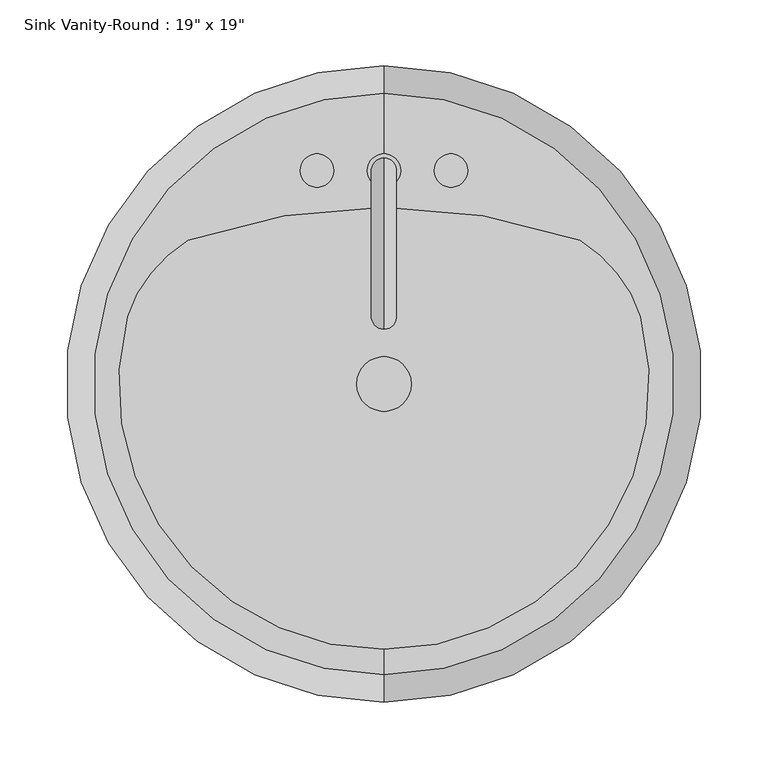
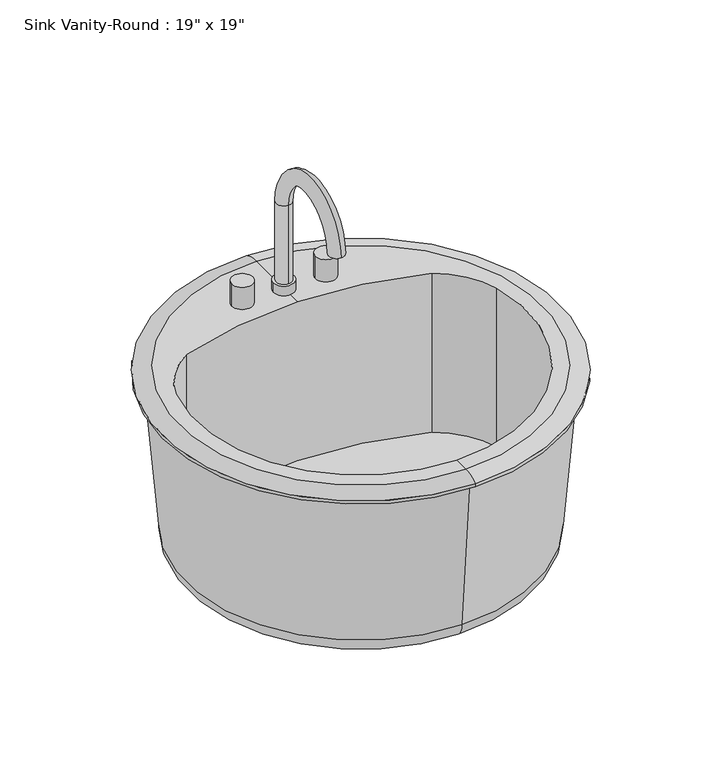
"""IFC4 building model written with IfcOpenShell, lengths in millimetres: flow terminal geometry."""

from ifc_helpers import new_model, si_unit, point, frame, frame_2d, origin, place, context, project, spatial, polyline, circle_curve, ellipse_curve, trimmed, segment, composite_curve, outline, extrude, source, transform, mapped, element, save
from ifc_brep_helpers import plane_surface, cylinder_surface, revolved_surface, advanced_brep


def flow_terminal_d49f872f(model_context):
    return source(origin(), model_context, "Body", "SolidModel", [
        advanced_brep(
        [(83.9517406, 247.0927185, 796.925), (109.3517406, 247.0927185, 796.925), (96.6517406, 237.5677185, 909.6375), (96.6517406, 256.6177185, 909.6375), (96.6517406, 256.6177185, 809.1602909), (96.6517406, 237.5677185, 809.1602909), (96.6517406, 145.7775038, 909.6375), (96.6517406, 126.7275038, 909.6375), (83.9517406, 247.0927185, 809.1602909), (109.3517406, 247.0927185, 809.1602909)],
        [
            (0, 1, circle_curve(frame((96.6517406, 247.0927185, 796.925), z_axis=(0.0, 0.0, -1.0), x_axis=(1.0, 0.0, 0.0)), 12.7)),
            (1, 0, circle_curve(frame((96.6517406, 247.0927185, 796.925), z_axis=(0.0, 0.0, -1.0), x_axis=(1.0, 0.0, 0.0)), 12.7)),
            (2, 3, circle_curve(frame((96.6517406, 247.0927185, 909.6375), z_axis=(0.0, 0.0, -1.0), x_axis=(0.0, 1.0, 0.0)), 9.525)),
            (3, 4),
            (4, 5, circle_curve(frame((96.6517406, 247.0927185, 809.1602909), z_axis=(0.0, 0.0, 1.0), x_axis=(0.0, 1.0, 0.0)), 9.525)),
            (5, 2),
            (3, 2, circle_curve(frame((96.6517406, 247.0927185, 909.6375), z_axis=(0.0, 0.0, -1.0), x_axis=(0.0, 1.0, 0.0)), 9.525)),
            (5, 4, circle_curve(frame((96.6517406, 247.0927185, 809.1602909), z_axis=(0.0, 0.0, 1.0), x_axis=(0.0, 1.0, 0.0)), 9.525)),
            (6, 7, circle_curve(frame((96.6517406, 136.2525038, 909.6375), z_axis=(0.0, 0.0, -1.0), x_axis=(0.0, -1.0, 0.0)), 9.525)),
            (7, 6, circle_curve(frame((96.6517406, 136.2525038, 909.6375), z_axis=(0.0, 0.0, -1.0), x_axis=(0.0, -1.0, 0.0)), 9.525)),
            (2, 6, circle_curve(frame((96.6517406, 191.6726112, 909.6375), z_axis=(1.0, 0.0, 0.0), x_axis=(0.0, 1.0, 0.0)), 45.8951073)),
            (7, 3, circle_curve(frame((96.6517406, 191.6726112, 909.6375), z_axis=(-1.0, 0.0, 0.0), x_axis=(0.0, 1.0, 0.0)), 64.9451073)),
            (8, 9, circle_curve(frame((96.6517406, 247.0927185, 809.1602909), z_axis=(0.0, 0.0, 1.0), x_axis=(1.0, 0.0, 0.0)), 12.7)),
            (9, 8, circle_curve(frame((96.6517406, 247.0927185, 809.1602909), z_axis=(0.0, 0.0, 1.0), x_axis=(1.0, 0.0, 0.0)), 12.7)),
            (8, 0),
            (1, 9),
        ],
        [
            plane_surface(frame((96.6517406, 237.5677185, 796.925), z_axis=(0.0, 0.0, -1.0), x_axis=(1.0, 0.0, 0.0))),
            cylinder_surface(frame((96.6517406, 247.0927185, 796.925), z_axis=(0.0, 0.0, -1.0), x_axis=(0.0, 1.0, 0.0)), 9.525),
            plane_surface(frame((96.6517406, 191.6726112, 909.6375), z_axis=(0.0, 0.0, -1.0), x_axis=(0.0, -1.0, 0.0))),
            revolved_surface(trimmed(ellipse_curve(frame((96.6517406, 247.0927185, 909.6375), z_axis=(0.0, 0.0, -1.0), x_axis=(0.0, 1.0, 0.0)), 9.525, 9.525), [point((96.6517406, 237.5677185, 909.6375))], [point((96.6517406, 256.6177185, 909.6375))], True, "CARTESIAN"), (96.6517406, 191.6726112, 909.6375), (1.0, 0.0, 0.0)),
            revolved_surface(trimmed(ellipse_curve(frame((96.6517406, 247.0927185, 909.6375), z_axis=(0.0, 0.0, -1.0), x_axis=(0.0, 1.0, 0.0)), 9.525, 9.525), [point((96.6517406, 256.6177185, 909.6375))], [point((96.6517406, 237.5677185, 909.6375))], True, "CARTESIAN"), (96.6517406, 191.6726112, 909.6375), (1.0, 0.0, 0.0)),
            plane_surface(frame((109.3517406, 247.0927185, 809.1602909), z_axis=(0.0, 0.0, 1.0), x_axis=(0.0, 1.0, 0.0))),
            cylinder_surface(frame((96.6517406, 247.0927185, 796.925), z_axis=(0.0, 0.0, 1.0), x_axis=(1.0, 0.0, 0.0)), 12.7),
        ],
        [
            (0, [[1, 2]]),
            (1, [[3, 4, 5, 6]]),
            (1, [[7, -6, 8, -4]]),
            (2, [[9, 10]]),
            (3, [[-3, 11, -10, 12]]),
            (4, [[-7, -12, -9, -11]]),
            (5, [[13, 14], [-5, -8]]),
            (6, [[-13, 15, -2, 16]]),
            (6, [[-14, -16, -1, -15]]),
        ],
    ),
        extrude(outline(composite_curve([segment(trimmed(circle_curve(frame_2d((45.8517406, 247.0927185)), 12.7), [point((33.1517406, 247.0927185))], [point((58.5517406, 247.0927185))], False, "CARTESIAN"), True, "CONTINUOUS"), segment(trimmed(circle_curve(frame_2d((45.8517406, 247.0927185)), 12.7), [point((58.5517406, 247.0927185))], [point((33.1517406, 247.0927185))], False, "CARTESIAN"), True, "CONTINUOUS")], self_intersect=False)), frame((0.0, 0.0, 796.925), z_axis=(0.0, 0.0, 1.0), x_axis=(1.0, 0.0, 0.0)), (0.0, 0.0, 1.0), 28.575),
        extrude(outline(composite_curve([segment(trimmed(circle_curve(frame_2d((147.4517406, 247.0927185)), 12.7), [point((134.7517406, 247.0927185))], [point((160.1517406, 247.0927185))], False, "CARTESIAN"), True, "CONTINUOUS"), segment(trimmed(circle_curve(frame_2d((147.4517406, 247.0927185)), 12.7), [point((160.1517406, 247.0927185))], [point((134.7517406, 247.0927185))], False, "CARTESIAN"), True, "CONTINUOUS")], self_intersect=False)), frame((0.0, 0.0, 796.925), z_axis=(0.0, 0.0, 1.0), x_axis=(1.0, 0.0, 0.0)), (0.0, 0.0, 1.0), 28.575),
        extrude(outline(composite_curve([segment(trimmed(circle_curve(frame_2d((96.6517406, 85.1677185)), 20.6375), [point((76.0142406, 85.1677185))], [point((117.2892406, 85.1677185))], False, "CARTESIAN"), True, "CONTINUOUS"), segment(trimmed(circle_curve(frame_2d((96.6517406, 85.1677185)), 20.6375), [point((117.2892406, 85.1677185))], [point((76.0142406, 85.1677185))], False, "CARTESIAN"), True, "CONTINUOUS")], self_intersect=False)), frame((0.0, 0.0, 571.5), z_axis=(0.0, 0.0, 1.0), x_axis=(1.0, 0.0, 0.0)), (0.0, 0.0, 1.0), 21.1842611),
        advanced_brep(
        [(96.6517406, -135.3870093, 796.925), (96.6517406, 305.7224463, 796.925), (96.6517406, 326.4677185, 791.36875), (96.6517406, -156.1322815, 791.36875), (96.6517406, -116.2405705, 796.925), (-98.1703414, 136.2525038, 796.925), (-52.1534933, 194.0861398, 796.925), (96.6517406, 219.2662048, 796.925), (245.4569744, 194.0861398, 796.925), (291.4738225, 136.2525038, 796.925), (96.6517406, -107.1264028, 571.5), (96.6517406, 277.4618398, 571.5), (96.6517406, 85.1677185, 571.5), (96.6517406, -127.6827361, 592.6842611), (96.6517406, 298.0181731, 592.6842611), (96.6517406, -144.2260315, 787.4), (96.6517406, 314.5614685, 787.4), (96.6517406, -156.1322815, 787.4), (96.6517406, 326.4677185, 787.4), (245.4569744, 194.0861398, 592.6842611), (-52.1534933, 194.0861398, 592.6842611), (-98.1703414, 136.2525038, 592.6842611), (291.4738225, 136.2525038, 592.6842611)],
        [
            (0, 1, circle_curve(frame((96.6517406, 85.1677185, 796.925), z_axis=(0.0, 0.0, -1.0), x_axis=(0.0, 1.0, 0.0)), 220.5547278)),
            (1, 2, circle_curve(frame((96.6517406, 309.4374616, 769.289434), z_axis=(-1.0, 0.0, 0.0), x_axis=(0.0, 1.0, 0.0)), 27.8841505)),
            (2, 3, circle_curve(frame((96.6517406, 85.1677185, 791.36875), z_axis=(0.0, 0.0, 1.0), x_axis=(0.0, 1.0, 0.0)), 241.3)),
            (3, 0, circle_curve(frame((96.6517406, -139.1020246, 769.289434), z_axis=(-1.0, 0.0, 0.0), x_axis=(0.0, -1.0, 0.0)), 27.8841505)),
            (1, 0, circle_curve(frame((96.6517406, 85.1677185, 796.925), z_axis=(0.0, 0.0, -1.0), x_axis=(0.0, 1.0, 0.0)), 220.5547278)),
            (3, 2, circle_curve(frame((96.6517406, 85.1677185, 791.36875), z_axis=(0.0, 0.0, 1.0), x_axis=(0.0, 1.0, 0.0)), 241.3)),
            (0, 4),
            (4, 5, circle_curve(frame((96.6517406, 85.1677185, 796.925), z_axis=(0.0, 0.0, -1.0), x_axis=(1.0, 0.0, 0.0)), 201.408289)),
            (5, 6, circle_curve(frame((1.3689689, 104.2755165, 796.925), z_axis=(0.0, 0.0, -1.0), x_axis=(1.0, 0.0, 0.0)), 104.5495194)),
            (6, 7, circle_curve(frame((96.6517406, -233.0168462, 796.925), z_axis=(0.0, 0.0, -1.0), x_axis=(1.0, 0.0, 0.0)), 452.283051)),
            (7, 1),
            (7, 8, circle_curve(frame((96.6517406, -233.0168462, 796.925), z_axis=(0.0, 0.0, -1.0), x_axis=(1.0, 0.0, 0.0)), 452.283051)),
            (8, 9, circle_curve(frame((191.9345122, 104.2755165, 796.925), z_axis=(0.0, 0.0, -1.0), x_axis=(1.0, 0.0, 0.0)), 104.5495194)),
            (9, 4, circle_curve(frame((96.6517406, 85.1677185, 796.925), z_axis=(0.0, 0.0, -1.0), x_axis=(1.0, 0.0, 0.0)), 201.408289)),
            (10, 11, circle_curve(frame((96.6517406, 85.1677185, 571.5), z_axis=(0.0, 0.0, -1.0), x_axis=(0.0, 1.0, 0.0)), 192.2941213)),
            (11, 12),
            (12, 10),
            (11, 10, circle_curve(frame((96.6517406, 85.1677185, 571.5), z_axis=(0.0, 0.0, -1.0), x_axis=(0.0, 1.0, 0.0)), 192.2941213)),
            (10, 13, circle_curve(frame((96.6517406, -107.1264028, 592.0656396), z_axis=(-1.0, 0.0, 0.0), x_axis=(0.0, -1.0, 0.0)), 20.5656396)),
            (13, 14, circle_curve(frame((96.6517406, 85.1677185, 592.6842611), z_axis=(0.0, 0.0, -1.0), x_axis=(0.0, 1.0, 0.0)), 212.8504546)),
            (14, 11, circle_curve(frame((96.6517406, 277.4618398, 592.0656396), z_axis=(-1.0, 0.0, 0.0), x_axis=(0.0, 1.0, 0.0)), 20.5656396)),
            (14, 13, circle_curve(frame((96.6517406, 85.1677185, 592.6842611), z_axis=(0.0, 0.0, -1.0), x_axis=(0.0, 1.0, 0.0)), 212.8504546)),
            (13, 15),
            (15, 16, circle_curve(frame((96.6517406, 85.1677185, 787.4), z_axis=(0.0, 0.0, -1.0), x_axis=(0.0, 1.0, 0.0)), 229.39375)),
            (16, 14),
            (16, 15, circle_curve(frame((96.6517406, 85.1677185, 787.4), z_axis=(0.0, 0.0, -1.0), x_axis=(0.0, 1.0, 0.0)), 229.39375)),
            (15, 17),
            (17, 18, circle_curve(frame((96.6517406, 85.1677185, 787.4), z_axis=(0.0, 0.0, -1.0), x_axis=(0.0, 1.0, 0.0)), 241.3)),
            (18, 16),
            (18, 17, circle_curve(frame((96.6517406, 85.1677185, 787.4), z_axis=(0.0, 0.0, -1.0), x_axis=(0.0, 1.0, 0.0)), 241.3)),
            (2, 18),
            (17, 3),
            (19, 20, circle_curve(frame((96.6517406, -233.0168462, 592.6842611), z_axis=(0.0, 0.0, 1.0), x_axis=(1.0, 0.0, 0.0)), 452.283051)),
            (20, 21, circle_curve(frame((1.3689689, 104.2755165, 592.6842611), z_axis=(0.0, 0.0, 1.0), x_axis=(1.0, 0.0, 0.0)), 104.5495194)),
            (21, 22, circle_curve(frame((96.6517406, 85.1677185, 592.6842611), z_axis=(0.0, 0.0, 1.0), x_axis=(1.0, 0.0, 0.0)), 201.408289)),
            (22, 19, circle_curve(frame((191.9345122, 104.2755165, 592.6842611), z_axis=(0.0, 0.0, 1.0), x_axis=(1.0, 0.0, 0.0)), 104.5495194)),
            (19, 8),
            (6, 20),
            (5, 21),
            (9, 22),
        ],
        [
            revolved_surface(trimmed(ellipse_curve(frame((96.6517406, 309.4374616, 769.289434), z_axis=(1.0, 0.0, 0.0), x_axis=(0.0, 1.0, 0.0)), 27.8841505, 27.8841505), [point((96.6517406, 326.4677185, 791.36875))], [point((96.6517406, 305.7224463, 796.925))], True, "CARTESIAN"), (96.6517406, 85.1677185, 796.925), (0.0, 0.0, 1.0)),
            plane_surface(frame((96.6517406, 85.1677185, 796.925), z_axis=(0.0, 0.0, 1.0), x_axis=(0.0, 1.0, 0.0))),
            plane_surface(frame((96.6517406, 85.1677185, 571.5), z_axis=(0.0, 0.0, -1.0), x_axis=(0.0, 1.0, 0.0))),
            revolved_surface(trimmed(ellipse_curve(frame((96.6517406, 277.4618398, 592.0656396), z_axis=(1.0, 0.0, 0.0), x_axis=(0.0, 1.0, 0.0)), 20.5656396, 20.5656396), [point((96.6517406, 277.4618398, 571.5))], [point((96.6517406, 298.0181731, 592.6842611))], True, "CARTESIAN"), (96.6517406, 85.1677185, 796.925), (0.0, 0.0, 1.0)),
            revolved_surface(polyline([(96.6517406, 298.0181731, 592.6842611), (96.6517406, 314.5614685, 787.4)]), (96.6517406, 85.1677185, 796.925), (0.0, 0.0, 1.0)),
            plane_surface(frame((96.6517406, 85.1677185, 787.4), z_axis=(0.0, 0.0, -1.0), x_axis=(0.0, 1.0, 0.0))),
            cylinder_surface(frame((96.6517406, 85.1677185, 796.925), z_axis=(0.0, 0.0, 1.0), x_axis=(0.0, 1.0, 0.0)), 241.3),
            plane_surface(frame((548.9347916, -233.0168462, 592.6842611), z_axis=(0.0, 0.0, 1.0), x_axis=(0.0, -1.0, 0.0))),
            revolved_surface(polyline([(548.9347916, -233.0168462, 796.925), (548.9347916, -233.0168462, 592.6842611)]), (96.6517406, -233.0168462, 592.6842611), (0.0, 0.0, 1.0)),
            revolved_surface(polyline([(105.91848829999999, 104.2755165, 796.925), (105.91848829999999, 104.2755165, 592.6842611)]), (1.3689689, 104.2755165, 592.6842611), (0.0, 0.0, 1.0)),
            revolved_surface(polyline([(298.0600296, 85.1677185, 796.925), (298.0600296, 85.1677185, 592.6842611)]), (96.6517406, 85.1677185, 592.6842611), (0.0, 0.0, 1.0)),
            revolved_surface(polyline([(296.4840316, 104.2755165, 796.925), (296.4840316, 104.2755165, 592.6842611)]), (191.9345122, 104.2755165, 592.6842611), (0.0, 0.0, 1.0)),
        ],
        [
            (0, [[1, 2, 3, 4]]),
            (0, [[-2, 5, -4, 6]]),
            (1, [[-1, 7, 8, 9, 10, 11]]),
            (1, [[-5, -11, 12, 13, 14, -7]]),
            (2, [[15, 16, 17]]),
            (2, [[-16, 18, -17]]),
            (3, [[-15, 19, 20, 21]]),
            (3, [[-18, -21, 22, -19]]),
            (4, [[-20, 23, 24, 25]]),
            (4, [[-22, -25, 26, -23]]),
            (5, [[-24, 27, 28, 29]]),
            (5, [[-26, -29, 30, -27]]),
            (6, [[-3, 31, -28, 32]]),
            (6, [[-6, -32, -30, -31]]),
            (7, [[33, 34, 35, 36]]),
            (8, [[-33, 37, -12, -10, 38]]),
            (9, [[-34, -38, -9, 39]]),
            (10, [[-35, -39, -8, -14, 40]]),
            (11, [[-36, -40, -13, -37]]),
        ],
    ),
    ])


if __name__ == "__main__":
    model = new_model("IFC4")
    model_context = context("Model", 3, world=origin())
    ifc_project = project(units=[si_unit("LENGTHUNIT", "METRE", prefix="MILLI")], contexts=[model_context])
    site = spatial("IfcSite", under=ifc_project)
    building = spatial("IfcBuilding", under=site)
    placement = place(None, origin())
    flow_terminal_shape = flow_terminal_d49f872f(model_context)
    element("IfcFlowTerminal", 1, ObjectType="Sink Vanity-Round : 19\" x 19\"", at=placement, inside=building, context=model_context, shape_type="MappedRepresentation", body=[
        mapped(flow_terminal_shape, transform((0.0, 0.0, 0.0), x_axis=(1.0, 0.0, 0.0), y_axis=(0.0, 1.0, 0.0), z_axis=(0.0, 0.0, 1.0))),
    ])
    save(model, "model.ifc")

# Revit data of these elements
# Type "Sink Vanity-Round : 19\" x 19\""
#   Assembly Code = "D2010400"
#   Top Of Counter = 2' - 7"
#   Basin Material = Porcelain, Linen
#   Faucet Material = Steel, Polished
#   Default Elevation = 0
# Element 1 (IfcFlowTerminal, "Sink Vanity-Round : 19\" x 19\"")
#   Materials on its faces: "Porcelain, Linen", "Steel, Polished"
# Materials
#   "Porcelain, Linen": class "Ceramic", colour RGB 249 239 230, transparency 0, Description = "Porcelain, linen", Cost = 0
#   "Steel, Polished": class "Metal", colour RGB 57 57 57, transparency 0, Description = "Polished steel", Cost = 0
